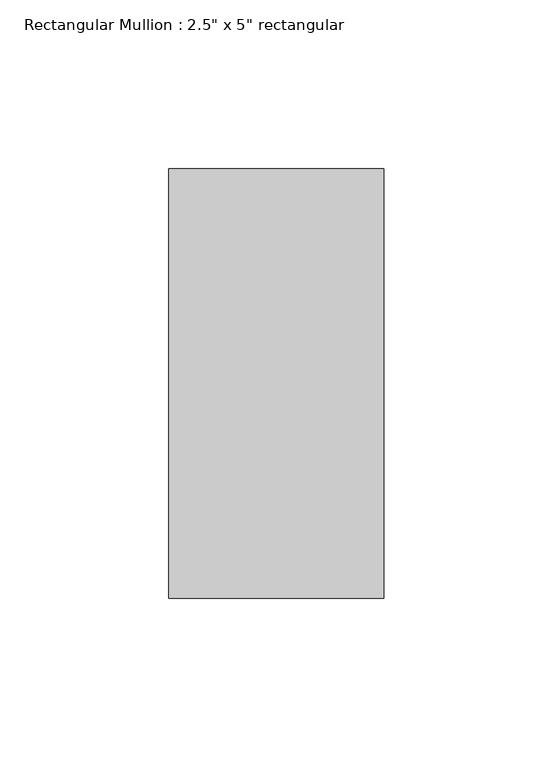
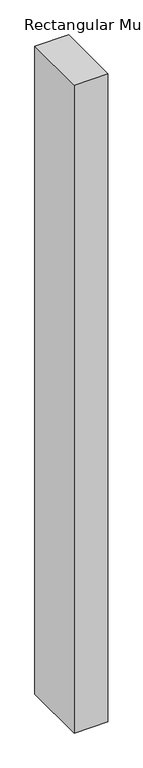
"""IFC4 building model written with IfcOpenShell, lengths in millimetres: member geometry."""

from ifc_helpers import new_model, si_unit, frame, origin, place, context, project, spatial, polyline, outline, extrude, source, transform, mapped, element, save


def member_54cb9db3(model_context):
    return source(origin(), model_context, "Body", "SweptSolid", [
        extrude(outline(polyline([(0.0, 63.5), (0.0, -63.5), (-63.5, -63.5), (-63.5, 63.5), (0.0, 63.5)])), frame((0.0, 0.0, -1282.852721), z_axis=(0.0, 0.0, 1.0), x_axis=(1.0, 0.0, 0.0)), (0.0, 0.0, 1.0), 1282.852721),
    ])


if __name__ == "__main__":
    model = new_model("IFC4")
    model_context = context("Model", 3, world=origin())
    ifc_project = project(units=[si_unit("LENGTHUNIT", "METRE", prefix="MILLI")], contexts=[model_context])
    site = spatial("IfcSite", under=ifc_project)
    building = spatial("IfcBuilding", under=site)
    placement = place(None, origin())
    member_shape = member_54cb9db3(model_context)
    element("IfcMember", 1, ObjectType="Rectangular Mullion : 2.5\" x 5\" rectangular", at=placement, inside=building, context=model_context, shape_type="MappedRepresentation", body=[
        mapped(member_shape, transform((0.0, 0.0, 0.0), x_axis=(1.0, 0.0, 0.0), y_axis=(0.0, 1.0, 0.0), z_axis=(0.0, 0.0, 1.0))),
    ])
    save(model, "model.ifc")

# Revit data of these elements
# Type "Rectangular Mullion : 2.5\" x 5\" rectangular"
#   built-in parameter 1007304 = 0.416667 (stored number, unit not read)
#   built-in parameter 1007301 = 0.104167 (stored number, unit not read)
#   built-in parameter 1007300 = 0.104167 (stored number, unit not read)
# Element 1 (IfcMember, "Rectangular Mullion : 2.5\" x 5\" rectangular")
#   Materials on its faces: "Aluminum"
# Materials
#   "Aluminum": class "Metal", colour RGB 247 247 247, transparency 0, Description = "Aluminum 6061", Cost = 0
